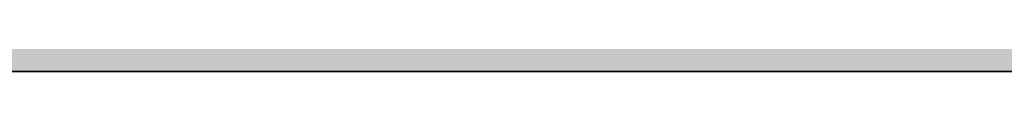
# Model space of a CAD drawing. Units: inches. Extents: x 2083 to 3317, y 1141 to 2115.
# Tile 150 of 256: x 3126.946713 to 3126.955939, y 1263.26136 to 1263.261503. Entities that reach past the tile are written whole.
import ezdxf

# ---------------------------------------------------------------- set-up
doc = ezdxf.new("R2010")
doc.units = ezdxf.units.IN
doc.layers.add('A-ANNO-DIMS', color=2, linetype='Continuous', lineweight=18)
doc.layers.add('A-WALL', color=7, linetype='Continuous', lineweight=35)
doc.layers.add('A-WALL-PATT', color=251, linetype='Continuous', lineweight=13, true_color=0x636466)
doc.styles.get("Standard").update_dxf_attribs({"font": 'arial.ttf'})
doc.dimstyles.new('ISO-25', dxfattribs={"dimtxt": 12, "dimasz": 12, "dimexe": 1.25, "dimexo": 0.625, "dimtad": 1, "dimlunit": 3, "dimtxsty": 'Standard', "dimcen": 2.5, "dimadec": 0, "dimazin": 0, "dimtfac": 1, "dimtmove": 0, "dimatfit": 3, "dimfxl": 1, "dimarcsym": 0})

# ---------------------------------------------------------------- blocks, each defined once
blk = doc.blocks.new('*D10')
at = {"layer": 'A-ANNO-DIMS', "color": 0, "lineweight": -2, "transparency": 16777216}
for p, q in [((2862.9597832, 1262.6363601), (2862.9597832, 1201.3844498)), ((3126.9597832, 1262.6363601), (3126.9597832, 1201.3844498)), ((2874.9597832, 1202.6344498), (3114.9597832, 1202.6344498))]:
    blk.add_line(p, q, dxfattribs=at)
at = {"layer": 'A-ANNO-DIMS', "color": 0, "transparency": 16777216}
for points in [[(2874.9597832, 1204.6344498), (2874.9597832, 1200.6344498), (2862.9597832, 1202.6344498)], [(3114.9597832, 1204.6344498), (3114.9597832, 1200.6344498), (3126.9597832, 1202.6344498)]]:
    blk.add_solid(points, dxfattribs=at)
at = {"layer": 'Defpoints', "color": 0, "transparency": 16777216}
for p in [(2862.9597832, 1263.2613601), (3126.9597832, 1263.2613601), (3126.9597832, 1202.6344498)]:
    blk.add_point(p, dxfattribs=at)
at = {"layer": 'A-ANNO-DIMS', "color": 0, "transparency": 16777216, "insert": (2994.9597832, 1209.2840064), "char_height": 12, "attachment_point": 5}
blk.add_mtext("22'", dxfattribs=at)

msp = doc.modelspace()

# ---------------------------------------------------------------- hatches: boundary and pattern name
at = {"layer": 'A-WALL-PATT'}
h = msp.add_hatch(color=256, dxfattribs=at)
h.dxf.hatch_style = 1
h.paths.add_polyline_path([(3126.9597832, 2020.7613601), (2748.9597832, 2020.7613601), (2604.9597832, 2020.7613601), (2226.9597832, 2020.7613601), (2226.9597832, 1702.7613601), (2466.9597832, 1702.7613601), (2466.9597832, 1582.7613601), (2418.9597832, 1582.7613601), (2418.9597832, 1477.7613601), (2226.9597832, 1477.7613601), (2226.9597832, 1263.2613601), (2544.9597832, 1263.2613601), (2544.9597832, 1411.7613601), (2604.9597832, 1411.7613601), (2685.9597832, 1411.7613601), (2685.9597832, 1420.7613601), (2604.9597832, 1420.7613601), (2604.9597832, 1573.7613601), (2604.9597832, 1702.7613601), (2604.9597832, 2011.7613601), (2748.9597832, 2011.7613601), (2748.9597832, 1702.7613601), (2862.9597832, 1702.7613601), (2862.9597832, 1621.7613601), (2871.9597832, 1621.7613601), (2871.9597832, 1702.7613601), (2883.9597832, 1702.7613601), (2883.9597832, 1706.9394595, -0.026459), (2883.9597832, 1711.7613601), (2757.9597832, 1711.7613601), (2757.9597832, 1807.7613601), (2787.9597832, 1807.7613601), (2787.9597832, 1812.2613601), (2757.9597832, 1812.2613601), (2757.9597832, 2011.7613601), (2877.9597832, 2011.7613601), (2877.9597832, 1812.2613601), (2847.9597832, 1812.2613601), (2847.9597832, 1807.7613601), (2889.8357425, 1807.7613601), (2889.8357425, 1812.2613601), (2882.4597832, 1812.2613601), (2882.4597832, 2011.7613601), (3117.9597832, 2011.7613601), (3117.9597832, 1812.2613601), (2937.8357425, 1812.2613601), (2937.8357425, 1807.7613601), (2995.7097832, 1807.7613601), (2995.7097832, 1796.1176655), (3000.2097832, 1796.1176655), (3000.2097832, 1807.7613601), (3117.9597832, 1807.7613601), (3117.9597832, 1711.7613601), (3000.2097832, 1711.7613601), (3000.2097832, 1760.1176655), (2998.5727047, 1760.1176655, -0.020711), (2995.7097832, 1760.1176655), (2995.7097832, 1711.7613601), (2931.9597832, 1711.7613601), (2931.9597832, 1702.7613601), (3126.9597832, 1702.7613601)])
h.paths.add_polyline_path([(2471.4597832, 2011.7613601), (2471.4597832, 1810.0113601), (2462.7169357, 1810.0113601), (2462.7169357, 1805.5113601), (2505.9597832, 1805.5113601), (2505.9597832, 1810.0113601), (2475.9597832, 1810.0113601), (2475.9597832, 2011.7613601), (2595.9597832, 2011.7613601), (2595.9597832, 1810.0113601), (2565.9597832, 1810.0113601), (2565.9597832, 1805.5113601), (2595.9597832, 1805.5113601), (2595.9597832, 1711.7613601), (2235.9597832, 1711.7613601), (2235.9597832, 1805.5113601), (2353.7097832, 1805.5113601), (2353.7097832, 1796.0541624), (2358.2097832, 1796.0541624), (2358.2097832, 1805.5113601), (2414.7169357, 1805.5113601), (2414.7169357, 1810.0113601), (2235.9597832, 1810.0113601), (2235.9597832, 2011.7613601)], flags=16)
h.paths.add_polyline_path([(2270.2047343, 1994.6100082), (2270.2047343, 1970.6100082), (2246.2047343, 1970.6100082), (2246.2047343, 1994.6100082)], flags=0)
edge = h.paths.add_edge_path(flags=0)
edge.add_ellipse((2332.027391, 1899.7981761), major_axis=(-3.0429938, 3.0429938), ratio=0.16825245, start_angle=-161.3321656, end_angle=-156.3071136, ccw=False)
edge.add_ellipse((2333.0820373, 1898.7435297), major_axis=(-1.0546463, 1.0546463), ratio=0.453532097, start_angle=-123.371019, end_angle=-94.1591066)
edge = h.paths.add_edge_path(flags=0)
edge.add_ellipse((2332.027391, 1968.8762897), major_axis=(3.0429938, 3.0429938), ratio=0.16825245, start_angle=18.6678344, end_angle=23.6928864)
edge.add_spline(control_points=[(2332.9255964, 1970.6911045), (2332.2267681, 1970.3360997), (2330.8937087, 1969.6589054), (2328.4130803, 1970.9321376), (2327.2039345, 1967.7487119), (2324.7095965, 1969.9555886), (2322.5328223, 1967.012354), (2320.0128462, 1971.2958124), (2317.6803077, 1968.1578449), (2316.0405263, 1967.1020468), (2315.4269045, 1966.8096022)], knot_values=[0, 0, 0, 0, 2.267059, 4.324559, 6.685584, 8.878641, 11.121502, 14.300359, 17.755284, 19.732645, 19.732645, 19.732645, 19.732645], degree=3, periodic=0)
edge.add_ellipse((2332.027391, 1968.8762897), major_axis=(3.0429938, 3.0429938), ratio=0.16825245, start_angle=18.6678344, end_angle=23.6928864, ccw=False)
edge.add_ellipse((2333.0820373, 1969.930936), major_axis=(1.0546463, 1.0546463), ratio=0.453532097, start_angle=56.628981, end_angle=85.8408934, ccw=False)
edge = h.paths.add_edge_path(flags=0)
edge.add_spline(control_points=[(2296.4282874, 1967.9879081), (2293.6278045, 1965.3363137), (2287.7036238, 1959.727094), (2299.7438601, 1949.9956993), (2294.5325909, 1935.6685275), (2290.5732281, 1920.6035119), (2293.3941244, 1909.9736911), (2296.1854073, 1904.9665431)], knot_values=[0.099185, 0.099185, 0.099185, 0.099185, 0.345301, 0.619822, 0.982653, 1.386093, 1.810555, 1.810555, 1.810555, 1.810555], degree=3, periodic=0)
edge.add_spline(control_points=[(2296.1854073, 1904.9665431), (2297.3835817, 1902.6193002), (2298.0009694, 1901.9493116), (2298.5529698, 1901.4681549)], knot_values=[0.006246, 0.006246, 0.006246, 0.006246, 0.055476, 0.055476, 0.055476, 0.055476], degree=3, periodic=0)
edge.add_spline(control_points=[(2298.5529698, 1901.4681549), (2297.2586121, 1900.9232238), (2295.2252939, 1900.2321257), (2293.0602287, 1900.6142053), (2292.1014227, 1900.788415), (2292.0895776, 1900.790568)], knot_values=[0.312835, 0.312835, 0.312835, 0.312835, 0.40178, 0.474987, 0.475903, 0.475903, 0.475903, 0.475903], degree=3, periodic=0)
edge.add_arc((2292.7936464, 1904.6641088), 3.9370079, 215.4208969, 259.6981795, ccw=False)
edge.add_spline(control_points=[(2289.5853139, 1902.3823039), (2289.4766524, 1902.5350874), (2289.3684805, 1902.6880353), (2289.2608648, 1902.8411699)], knot_values=[0.102872, 0.102872, 0.102872, 0.102872, 0.116896, 0.116896, 0.116896, 0.116896], degree=3, periodic=0)
edge.add_spline(control_points=[(2289.2608648, 1902.8411699), (2288.6866042, 1902.5501922), (2287.6400477, 1902.0199025), (2285.8813368, 1901.8739536), (2283.8529717, 1901.5043521), (2281.7199871, 1899.7105375), (2278.4669913, 1899.492942), (2276.1571361, 1901.8832022), (2272.2589526, 1899.8040711), (2267.7776054, 1901.8431828), (2262.2438819, 1900.1840326), (2257.414927, 1901.7820606), (2254.318374, 1900.7261196), (2253.1782849, 1900.3373431)], knot_values=[0, 0, 0, 0, 1.907977, 3.477176, 5.261074, 7.972851, 11.680248, 13.717921, 16.939592, 22.789562, 27.502503, 33.595215, 37.145618, 37.145618, 37.145618, 37.145618], degree=3, periodic=0)
edge.add_line((2253.1782849, 1900.3373431), (2250.2442397, 1902.8411699))
edge.add_line((2250.2442397, 1902.8411699), (2250.2442397, 1965.8332959))
edge.add_line((2250.2442397, 1965.8332959), (2253.1782849, 1968.3371226))
edge.add_spline(control_points=[(2253.1782849, 1968.3371226), (2254.318374, 1967.9483462), (2257.414927, 1966.8924051), (2262.2438819, 1968.4904332), (2267.7776054, 1966.8312829), (2271.5267301, 1968.5372172), (2273.8759143, 1967.8282895), (2274.2067012, 1967.7276424)], knot_values=[0, 0, 0, 0, 0.09018, 0.244935, 0.364644, 0.513233, 0.537855, 0.537855, 0.537855, 0.537855], degree=3, periodic=0)
edge.add_arc((2274.3528869, 1963.7933495), 3.9370079, 72.0511336, 92.1279492, ccw=False)
edge.add_arc((2281.2969331, 1985.2300027), 18.5962982, 252.05113361, 288.56572166)
edge.add_arc((2292.3167172, 1956.0288805), 12.6460805, 71.02678788, 113.77821843, ccw=False)
edge = h.paths.add_edge_path(flags=0)
edge.add_spline(control_points=[(2274.8994147, 1951.8561946), (2275.066156, 1951.6165924), (2275.2326866, 1951.3765878), (2275.3979871, 1951.1358545)], knot_values=[1.409916, 1.409916, 1.409916, 1.409916, 1.43159, 1.43159, 1.43159, 1.43159], degree=3, periodic=0)
edge.add_spline(control_points=[(2275.3979871, 1951.1358545), (2275.7921055, 1950.5618854), (2276.1792311, 1949.9837745), (2276.5455462, 1949.3971029)], knot_values=[1.358238, 1.358238, 1.358238, 1.358238, 1.409916, 1.409916, 1.409916, 1.409916], degree=3, periodic=0)
edge.add_line((2276.5455462, 1949.3971029), (2277.437289, 1947.8621847))
edge.add_spline(control_points=[(2277.437289, 1947.8621847), (2276.3038341, 1945.6731147), (2274.6396979, 1942.4268817), (2274.631615, 1938.0938998), (2272.7991237, 1930.8515498), (2274.3564261, 1943.8970461), (2275.9476814, 1947.9233558), (2276.5455462, 1949.3971029)], knot_values=[0.005632, 0.005632, 0.005632, 0.005632, 0.186014, 0.266002, 0.357087, 0.59639, 0.739732, 0.739732, 0.739732, 0.739732], degree=3, periodic=0)
edge.add_spline(control_points=[(2276.5455462, 1949.3971029), (2276.1792311, 1949.9837745), (2275.7921055, 1950.5618854), (2275.3979871, 1951.1358545)], knot_values=[1.358238, 1.358238, 1.358238, 1.358238, 1.409916, 1.409916, 1.409916, 1.409916], degree=3, periodic=0)
edge.add_spline(control_points=[(2275.3979871, 1951.1358545), (2274.9425002, 1950.0804523), (2274.2077604, 1948.0252718), (2273.9346018, 1944.8514774), (2272.4685341, 1937.6274891), (2273.4662155, 1945.6964663), (2274.7006154, 1951.0594725), (2274.8994147, 1951.8561946)], knot_values=[0.104364, 0.104364, 0.104364, 0.104364, 0.189636, 0.269624, 0.36071, 0.600013, 0.644622, 0.644622, 0.644622, 0.644622], degree=3, periodic=0)
h.paths.add_polyline_path([(2269.1675139, 1963.1275729, -0.357527), (2268.170633, 1960.9763695, -0.092561), (2268.170633, 1939.4363249, -0.357527), (2269.1675139, 1937.2851215, -0.357527), (2267.0163105, 1938.2820024, -0.164785), (2254.6855813, 1938.2820024, -0.357527), (2252.5343779, 1937.2851215, -0.357527), (2253.5312587, 1939.4363249, -0.092561), (2253.5312587, 1960.9763695, -0.357527), (2252.5343779, 1963.1275729, -0.357527), (2254.6855813, 1962.130692, -0.164785), (2267.0163105, 1962.130692, -0.357527)], flags=0)
h.paths.add_polyline_path([(2248.8740679, 1967.8017998), (2248.8740679, 1957.0277095), (2249.4577833, 1957.0277095), (2249.4577833, 1911.6467562), (2248.8740679, 1911.6467562), (2248.8740679, 1900.8726659), (2246.5118632, 1900.8726659, 0.197327), (2244.1496584, 1902.4568734), (2244.1496584, 1966.2175923, 0.197327), (2246.5118632, 1967.8017998)], flags=0)
h.paths.add_polyline_path([(2269.1675139, 1931.3893442, -0.357527), (2268.170633, 1929.2381408, -0.092561), (2268.170633, 1907.6980962, -0.357527), (2269.1675139, 1905.5468928, -0.357527), (2267.0163105, 1906.5437737, -0.164785), (2254.6855813, 1906.5437737, -0.357527), (2252.5343779, 1905.5468928, -0.357527), (2253.5312587, 1907.6980962, -0.092561), (2253.5312587, 1929.2381408, -0.357527), (2252.5343779, 1931.3893442, -0.357527), (2254.6855813, 1930.3924634, -0.164785), (2267.0163105, 1930.3924634, -0.357527)], flags=0)
edge = h.paths.add_edge_path(flags=0)
edge.add_spline(control_points=[(2276.1968578, 1906.7237016), (2276.1681442, 1909.0289278), (2276.1140492, 1913.371852), (2270.5984171, 1924.9249783), (2273.9051746, 1919.0127787), (2275.9217115, 1916.2620626), (2275.4745699, 1912.4021495), (2277.2578735, 1910.3806206), (2276.6960436, 1908.2250358), (2276.6462176, 1906.8130226), (2276.6178249, 1906.0084068)], knot_values=[0, 0, 0, 0, 8.61026, 16.221274, 18.843057, 23.804898, 27.440828, 29.356102, 31.203478, 33.650687, 33.650687, 33.650687, 33.650687], degree=3, periodic=0)
edge.add_spline(control_points=[(2276.6178249, 1906.0084068), (2276.6233131, 1905.6241436), (2276.4977381, 1904.6286608), (2275.4417789, 1903.8547251), (2274.9373144, 1903.0804497), (2274.8590804, 1902.8411699)], knot_values=[0.156488, 0.156488, 0.156488, 0.156488, 0.184398, 0.231376, 0.250598, 0.250598, 0.250598, 0.250598], degree=3, periodic=0)
edge.add_line((2274.8590804, 1902.8411699), (2276.50598, 1902.8411699))
edge.add_spline(control_points=[(2276.50598, 1902.8411699), (2276.7883084, 1903.0849395), (2277.6650711, 1904.1251958), (2278.2495378, 1904.340738), (2277.6538719, 1908.5273866), (2278.15567, 1906.2278078), (2278.100464, 1905.2859484), (2278.8466748, 1904.0690054), (2277.8567853, 1903.4149482), (2277.8741909, 1902.9910497), (2277.9035616, 1902.8411699)], knot_values=[0.059574, 0.059574, 0.059574, 0.059574, 0.080753, 0.103741, 0.16972, 0.176036, 0.207137, 0.240474, 0.262341, 0.27366, 0.27366, 0.27366, 0.27366], degree=3, periodic=0)
edge.add_line((2277.9035616, 1902.8411699), (2280.0298255, 1902.8411699))
edge.add_spline(control_points=[(2280.0298255, 1902.8411699), (2279.8882214, 1903.088398), (2279.4992571, 1903.9815512), (2280.1522839, 1905.9393491), (2278.103615, 1909.6577572), (2279.7623946, 1907.185285), (2280.3279002, 1904.8748608), (2280.4851086, 1903.4895904), (2281.4632687, 1903.2494323), (2281.7583431, 1902.9364967), (2281.8340361, 1902.8411699)], knot_values=[0.013856, 0.013856, 0.013856, 0.013856, 0.034874, 0.088867, 0.107879, 0.126738, 0.158714, 0.193757, 0.217487, 0.226722, 0.226722, 0.226722, 0.226722], degree=3, periodic=0)
edge.add_spline(control_points=[(2281.8340361, 1902.8411699), (2281.7875348, 1902.8267029), (2281.6470224, 1902.7829881), (2281.3955272, 1902.85949), (2281.088077, 1902.9852418), (2280.7206826, 1903.060902), (2280.3334513, 1903.0257257), (2280.1247668, 1902.898879), (2280.0298255, 1902.8411699)], knot_values=[0, 0, 0, 0, 0.14413, 0.435517, 0.749276, 1.153046, 1.548371, 1.878348, 1.878348, 1.878348, 1.878348], degree=3, periodic=0)
edge.add_line((2280.0298255, 1902.8411699), (2277.9035616, 1902.8411699))
edge.add_spline(control_points=[(2277.9035616, 1902.8411699), (2277.892855, 1902.7958553), (2277.865396, 1902.6796374), (2277.6074793, 1902.6874828), (2277.2740503, 1902.8006999), (2276.8379209, 1902.6197745), (2276.5838074, 1902.7892611), (2276.50598, 1902.8411699)], knot_values=[0, 0, 0, 0, 0.127189, 0.326199, 0.628009, 1.24357, 1.515331, 1.515331, 1.515331, 1.515331], degree=3, periodic=0)
edge.add_line((2276.50598, 1902.8411699), (2274.8590804, 1902.8411699))
edge.add_spline(control_points=[(2274.8590804, 1902.8411699), (2274.8144367, 1902.8985868), (2274.7251297, 1903.013446), (2274.4934765, 1903.1189684), (2274.2442854, 1902.9605386), (2273.9371207, 1903.1849416), (2273.6140395, 1902.9831428), (2273.4083164, 1902.8830449), (2273.322254, 1902.8411699)], knot_values=[0, 0, 0, 0, 0.21843, 0.436957, 0.687977, 0.990379, 1.398396, 1.69185, 1.69185, 1.69185, 1.69185], degree=3, periodic=0)
edge.add_spline(control_points=[(2273.322254, 1902.8411699), (2273.6167403, 1903.445692), (2274.2739977, 1904.5382529), (2276.0272387, 1904.5737017), (2276.2069634, 1906.5836372), (2276.1968578, 1906.7237016)], knot_values=[0.012227, 0.012227, 0.012227, 0.012227, 0.059472, 0.106218, 0.134458, 0.134458, 0.134458, 0.134458], degree=3, periodic=0)
h.paths.add_polyline_path([(2270.7760538, 1897.7898284), (2270.7760538, 1873.7898284), (2246.7760538, 1873.7898284), (2246.7760538, 1897.7898284)], flags=0)
h.paths.add_polyline_path([(2353.7097832, 1760.0050593), (2353.7097832, 1760.0541624), (2358.2097832, 1760.0541624, -0.033729)], flags=0)
h.paths.add_polyline_path([(2321.8191188, 1737.5291862), (2341.9953271, 1737.5291862, -0.414214), (2343.2032727, 1736.3212406), (2343.2032727, 1721.0205964, -0.414214), (2341.9953271, 1719.8126508), (2321.8191188, 1719.8126508, -0.414214), (2320.6111732, 1721.0205964), (2320.6111732, 1736.3212406, -0.414214)], flags=0)
h.paths.add_polyline_path([(2324.2350099, 1736.3212406), (2339.5794359, 1736.3212406, -0.414214), (2341.9953271, 1733.9053494), (2341.9953271, 1725.4497302, -0.414214), (2339.5794359, 1723.033839), (2333.6805885, 1723.033839), (2333.8453172, 1722.0454666, -0.870646), (2335.4253988, 1721.8258934, -0.767327), (2333.922694, 1721.4232449), (2331.2910241, 1721.4232449, -0.767327), (2329.7883193, 1721.8258934, -0.870646), (2331.3684009, 1722.0454666), (2331.5331296, 1723.033839), (2324.2350099, 1723.033839, -0.414214), (2321.8191188, 1725.4497302), (2321.8191188, 1733.9053494, -0.414214)], flags=0)
h.paths.add_polyline_path([(2570.4837892, 1928.6154443), (2589.6837892, 1928.6154443), (2590.1688286, 1928.6154443), (2590.1688286, 1904.9933971), (2570.4837892, 1904.9933971)], flags=0)
h.paths.add_polyline_path([(2574.4473242, 1927.2638215, -1), (2572.8288357, 1927.2638215, -1)], flags=0)
h.paths.add_polyline_path([(2573.0898665, 1926.9408768), (2573.925032, 1927.7760423), (2574.1477428, 1927.5533315), (2573.3125773, 1926.718166)], flags=0)
h.paths.add_polyline_path([(2578.7790648, 1919.7296175, -1), (2571.5916632, 1919.7296175, -1)], flags=0)
h.paths.add_polyline_path([(2578.385364, 1919.7296175, -1), (2571.985364, 1919.7296175, -1)], flags=0)
h.paths.add_polyline_path([(2331.5957638, 1729.4762156, -1), (2333.6179542, 1729.4762156, -1)], flags=0)
h.paths.add_polyline_path([(2578.0342282, 1927.2638215, -1), (2576.4157396, 1927.2638215, -1)], flags=0)
h.paths.add_polyline_path([(2576.6888513, 1927.5310886), (2576.9115621, 1927.7537993), (2577.7467276, 1926.9186339), (2577.5240168, 1926.6959231)], flags=0)
h.paths.add_polyline_path([(2578.1390648, 1909.8595388, -1), (2572.2316632, 1909.8595388, -1)], flags=0)
h.paths.add_polyline_path([(2577.745364, 1909.8595388, -1), (2572.625364, 1909.8595388, -1)], flags=0)
h.paths.add_polyline_path([(2583.7977179, 1927.2638215, -1), (2582.1792294, 1927.2638215, -1)], flags=0)
h.paths.add_polyline_path([(2582.7186487, 1927.7537993), (2583.5538142, 1926.9186339), (2583.3311034, 1926.6959231), (2582.4959379, 1927.5310886)], flags=0)
h.paths.add_polyline_path([(2582.4959379, 1927.5310886), (2582.7186487, 1927.7537993), (2583.5538142, 1926.9186339), (2583.3311034, 1926.6959231)], flags=0)
h.paths.add_polyline_path([(2587.7390648, 1920.5296175, -1), (2581.8316632, 1920.5296175, -1)], flags=0)
h.paths.add_polyline_path([(2587.345364, 1920.5296175, -1), (2582.225364, 1920.5296175, -1)], flags=0)
h.paths.add_polyline_path([(2587.3846219, 1927.2638215, -1), (2585.7661333, 1927.2638215, -1)], flags=0)
h.paths.add_polyline_path([(2586.0819925, 1926.9802469), (2586.917158, 1927.8154124), (2587.1398688, 1927.5927016), (2586.3047033, 1926.7575361)], flags=0)
h.paths.add_polyline_path([(2588.3790648, 1910.6595388, -1), (2581.1916632, 1910.6595388, -1)], flags=0)
h.paths.add_polyline_path([(2587.985364, 1910.6595388, -1), (2581.585364, 1910.6595388, -1)], flags=0)
h.paths.add_polyline_path([(2417.1677288, 1729.4778955), (2437.3439372, 1729.4778955, -0.414214), (2438.5518828, 1728.2699499), (2438.5518828, 1712.9693057, -0.414214), (2437.3439372, 1711.7613601), (2417.1677288, 1711.7613601, -0.414214), (2415.9597832, 1712.9693057), (2415.9597832, 1728.2699499, -0.414214)], flags=0)
h.paths.add_polyline_path([(2419.58362, 1728.2699499), (2434.928046, 1728.2699499, -0.414214), (2437.3439372, 1725.8540587), (2437.3439372, 1717.3984395, -0.414214), (2434.928046, 1714.9825483), (2429.0291985, 1714.9825483), (2429.1939273, 1713.9941758, -0.870646), (2430.7740089, 1713.7746027, -0.767327), (2429.2713041, 1713.3719542), (2426.6396342, 1713.3719542, -0.767327), (2425.1369294, 1713.7746027, -0.870646), (2426.717011, 1713.9941758), (2426.8817397, 1714.9825483), (2419.58362, 1714.9825483, -0.414214), (2417.1677288, 1717.3984395), (2417.1677288, 1725.8540587, -0.414214)], flags=0)
h.paths.add_polyline_path([(2419.58362, 1728.2699499), (2434.928046, 1728.2699499, -0.414214), (2437.3439372, 1725.8540587), (2437.3439372, 1717.3984395, -0.414214), (2434.928046, 1714.9825483), (2429.0291985, 1714.9825483), (2428.3581177, 1719.0090337), (2427.5528206, 1719.0090337), (2426.8817397, 1714.9825483), (2419.58362, 1714.9825483, -0.414214), (2417.1677288, 1717.3984395), (2417.1677288, 1725.8540587, -0.414214)], flags=0)
h.paths.add_polyline_path([(2426.9443739, 1721.4249248, -1), (2428.9665643, 1721.4249248, -1)], flags=0)
h.paths.add_polyline_path([(2475.9597832, 1702.7613601), (2595.9597832, 1702.7613601), (2595.9597832, 1582.7613601), (2475.9597832, 1582.7613601)], flags=16)
h.paths.add_polyline_path([(2427.9597832, 1573.7613601), (2595.9597832, 1573.7613601), (2595.9597832, 1468.7613601), (2595.9597832, 1420.7613601), (2384.4597832, 1420.7613601), (2384.4597832, 1468.7613601), (2427.9597832, 1468.7613601)], flags=16)
h.paths.add_polyline_path([(2379.9597832, 1468.7613601), (2379.9597832, 1420.7613601), (2235.9597832, 1420.7613601), (2235.9597832, 1468.7613601)], flags=16)
h.paths.add_polyline_path([(2317.8159962, 1466.695767), (2337.9922045, 1466.695767, -0.414214), (2339.2001501, 1465.4878214), (2339.2001501, 1450.1871771, -0.414214), (2337.9922045, 1448.9792315), (2317.8159962, 1448.9792315, -0.414214), (2316.6080506, 1450.1871771), (2316.6080506, 1465.4878214, -0.414214)], flags=0)
h.paths.add_polyline_path([(2320.2318874, 1465.4878214), (2335.5763133, 1465.4878214, -0.414214), (2337.9922045, 1463.0719302), (2337.9922045, 1454.616311, -0.414214), (2335.5763133, 1452.2004198), (2329.6774659, 1452.2004198), (2329.8421946, 1451.2120473, -0.870646), (2331.4222762, 1450.9924742, -0.767327), (2329.9195714, 1450.5898257), (2327.2879015, 1450.5898257, -0.767327), (2325.7851967, 1450.9924742, -0.870646), (2327.3652783, 1451.2120473), (2327.530007, 1452.2004198), (2320.2318874, 1452.2004198, -0.414214), (2317.8159962, 1454.616311), (2317.8159962, 1463.0719302, -0.414214)], flags=0)
h.paths.add_polyline_path([(2320.2318874, 1465.4878214), (2335.5763133, 1465.4878214, -0.414214), (2337.9922045, 1463.0719302), (2337.9922045, 1454.616311, -0.414214), (2335.5763133, 1452.2004198), (2329.6774659, 1452.2004198), (2329.006385, 1456.2269051), (2328.2010879, 1456.2269051), (2327.530007, 1452.2004198), (2320.2318874, 1452.2004198, -0.414214), (2317.8159962, 1454.616311), (2317.8159962, 1463.0719302, -0.414214)], flags=0)
h.paths.add_polyline_path([(2327.5926413, 1458.6427963, -1), (2329.6148317, 1458.6427963, -1)], flags=0)
h.paths.add_polyline_path([(2244.4117436, 1433.3404531), (2241.9209449, 1433.3404531, -0.414214), (2240.0178562, 1435.2435418), (2240.0178562, 1440.9528078, -0.414211), (2241.920925, 1442.8558965), (2244.4117436, 1442.8558965, -1.976472)], flags=0)
h.paths.add_polyline_path([(2245.3568884, 1434.3975358, -0.414214), (2245.3568884, 1441.7988138, -2.144098)], flags=0)
h.paths.add_polyline_path([(2535.9597832, 1416.2613601), (2535.9597832, 1272.2613601), (2235.9597832, 1272.2613601), (2235.9597832, 1416.2613601)], flags=16)
h.paths.add_polyline_path([(2260.1195614, 1384.2928413), (2260.1195614, 1362.0386487), (2237.8653688, 1362.0386487), (2237.8653688, 1384.2928413)], flags=0)
edge = h.paths.add_edge_path(flags=0)
edge.add_line((2318.2518466, 1362.0932983), (2318.1457968, 1362.0009726))
edge.add_ellipse((2317.4451158, 1360.4310442), major_axis=(2.8216404, 2.8216404), ratio=0.16825245, start_angle=18.6678344, end_angle=20.9481273, ccw=False)
edge.add_ellipse((2318.4230451, 1361.4089735), major_axis=(0.9779293, 0.9779293), ratio=0.453532097, start_angle=56.628981, end_angle=70.2262012, ccw=False)
edge = h.paths.add_edge_path(flags=0)
edge.add_line((2319.1073699, 1295.5710784), (2319.0150442, 1295.6771282))
edge.add_ellipse((2317.4451158, 1296.3778091), major_axis=(-2.8216404, 2.8216404), ratio=0.16825245, start_angle=-161.3321656, end_angle=-159.0518727, ccw=False)
edge.add_ellipse((2318.4230451, 1295.3998798), major_axis=(-0.9779293, 0.9779293), ratio=0.453532097, start_angle=-123.371019, end_angle=-109.7737988)
edge = h.paths.add_edge_path(flags=0)
edge.add_spline(control_points=[(2284.2103489, 1301.1702189), (2284.5806878, 1300.444719), (2284.8911891, 1299.8920243), (2285.159553, 1299.4610182)], knot_values=[0.039066, 0.039066, 0.039066, 0.039066, 0.055476, 0.055476, 0.055476, 0.055476], degree=3, periodic=0)
edge.add_line((2285.159553, 1299.4610182), (2284.2103489, 1301.1702189))
edge = h.paths.add_edge_path(flags=0)
edge.add_line((2280.4124579, 1297.2980125), (2283.3699905, 1297.0361216))
edge.add_line((2283.3699905, 1297.0361216), (2286.4056902, 1297.9263104))
edge.add_spline(control_points=[(2286.4056902, 1297.9263104), (2285.305487, 1297.4631193), (2284.3447774, 1297.1291508), (2283.3699905, 1297.0361216)], knot_values=[0.394369, 0.394369, 0.394369, 0.394369, 0.475903, 0.475903, 0.475903, 0.475903], degree=3, periodic=0)
edge.add_spline(control_points=[(2283.3699905, 1297.0361216), (2283.2813895, 1297.027666), (2282.316289, 1296.9573356), (2281.3125019, 1297.1344787), (2280.4234414, 1297.2960161), (2280.4124579, 1297.2980125)], knot_values=[0.312835, 0.312835, 0.312835, 0.312835, 0.320246, 0.393453, 0.394369, 0.394369, 0.394369, 0.394369], degree=3, periodic=0)
edge = h.paths.add_edge_path(flags=0)
edge.add_line((2284.4355615, 1359.6072854), (2280.4462909, 1355.328047))
edge.add_line((2280.4462909, 1355.328047), (2279.5799868, 1351.0177544))
edge.add_line((2279.5799868, 1351.0177544), (2282.4129737, 1346.5804327))
edge.add_spline(control_points=[(2282.4129737, 1346.5804327), (2283.1533308, 1345.5892358), (2284.2528957, 1344.0288973), (2284.801037, 1342.3871671), (2284.9351625, 1341.8055443)], knot_values=[1.240098, 1.240098, 1.240098, 1.240098, 1.332892, 1.382712, 1.382712, 1.382712, 1.382712], degree=3, periodic=0)
edge.add_spline(control_points=[(2284.9351625, 1341.8055443), (2285.3191079, 1340.1406002), (2285.2330291, 1338.4092041), (2284.9099384, 1336.6541222)], knot_values=[1.097484, 1.097484, 1.097484, 1.097484, 1.240098, 1.240098, 1.240098, 1.240098], degree=3, periodic=0)
edge.add_spline(control_points=[(2284.9099384, 1336.6541222), (2284.5868478, 1334.8990403), (2284.0267453, 1333.1202725), (2283.4626437, 1331.3605849)], knot_values=[0.95487, 0.95487, 0.95487, 0.95487, 1.097484, 1.097484, 1.097484, 1.097484], degree=3, periodic=0)
edge.add_line((2283.4626437, 1331.3605849), (2281.8903759, 1326.153357))
edge.add_line((2281.8903759, 1326.153357), (2280.7562592, 1321.0560888))
edge.add_line((2280.7562592, 1321.0560888), (2280.2992048, 1316.0019772))
edge.add_line((2280.2992048, 1316.0019772), (2280.7159327, 1310.9500678))
edge.add_line((2280.7159327, 1310.9500678), (2282.0280939, 1305.9721367))
edge.add_line((2282.0280939, 1305.9721367), (2284.2103489, 1301.1702189))
edge.add_spline(control_points=[(2284.2103489, 1301.1702189), (2283.3407305, 1302.7301854), (2282.6119044, 1304.3364933), (2282.0280939, 1305.9721367)], knot_values=[0.099185, 0.099185, 0.099185, 0.099185, 0.241799, 0.241799, 0.241799, 0.241799], degree=3, periodic=0)
edge.add_spline(control_points=[(2282.0280939, 1305.9721367), (2281.4442835, 1307.6077801), (2281.0054886, 1309.2727591), (2280.7159327, 1310.9500678)], knot_values=[0.241799, 0.241799, 0.241799, 0.241799, 0.384413, 0.384413, 0.384413, 0.384413], degree=3, periodic=0)
edge.add_spline(control_points=[(2280.7159327, 1310.9500678), (2280.4332411, 1312.5876134), (2280.2893863, 1314.2769594), (2280.2988938, 1315.9620324), (2280.2992048, 1316.0019772)], knot_values=[0.384413, 0.384413, 0.384413, 0.384413, 0.523647, 0.527028, 0.527028, 0.527028, 0.527028], degree=3, periodic=0)
edge.add_spline(control_points=[(2280.2992048, 1316.0019772), (2280.3123257, 1317.6869552), (2280.4778706, 1319.3679256), (2280.7562592, 1321.0560888)], knot_values=[0.527028, 0.527028, 0.527028, 0.527028, 0.669642, 0.669642, 0.669642, 0.669642], degree=3, periodic=0)
edge.add_spline(control_points=[(2280.7562592, 1321.0560888), (2281.0346478, 1322.7442519), (2281.4258801, 1324.4396079), (2281.8903759, 1326.153357)], knot_values=[0.669642, 0.669642, 0.669642, 0.669642, 0.812256, 0.812256, 0.812256, 0.812256], degree=3, periodic=0)
edge.add_spline(control_points=[(2281.8903759, 1326.153357), (2282.2643834, 1327.5332507), (2282.7878702, 1329.2618097), (2283.352751, 1331.0177803), (2283.4626437, 1331.3605849)], knot_values=[0.812256, 0.812256, 0.812256, 0.812256, 0.927087, 0.95487, 0.95487, 0.95487, 0.95487], degree=3, periodic=0)
edge.add_line((2283.4626437, 1331.3605849), (2284.9099384, 1336.6541222))
edge.add_line((2284.9099384, 1336.6541222), (2284.9351625, 1341.8055443))
edge.add_line((2284.9351625, 1341.8055443), (2282.4129737, 1346.5804327))
edge.add_spline(control_points=[(2282.4129737, 1346.5804327), (2281.2751273, 1348.1037918), (2280.0784467, 1349.5703178), (2279.5799868, 1351.0177544)], knot_values=[1.382712, 1.382712, 1.382712, 1.382712, 1.525326, 1.525326, 1.525326, 1.525326], degree=3, periodic=0)
edge.add_spline(control_points=[(2279.5799868, 1351.0177544), (2279.4432818, 1351.4147209), (2279.1363124, 1352.856922), (2279.7351897, 1354.2903851), (2280.4462909, 1355.328047)], knot_values=[1.525326, 1.525326, 1.525326, 1.525326, 1.564439, 1.667941, 1.667941, 1.667941, 1.667941], degree=3, periodic=0)
edge.add_spline(control_points=[(2280.4462909, 1355.328047), (2281.4261132, 1356.7578354), (2282.9308373, 1358.1825604), (2284.4355615, 1359.6072854)], knot_values=[1.667941, 1.667941, 1.667941, 1.667941, 1.810555, 1.810555, 1.810555, 1.810555], degree=3, periodic=0)
edge.add_arc((2280.6230749, 1348.518181), 11.7261796, 71.02678788, 113.77821843)
edge.add_arc((2270.4048917, 1375.5951559), 17.2435667, 252.05113361, 288.56572166, ccw=False)
edge.add_arc((2263.9659692, 1355.7178471), 3.6506221, 72.0511336, 92.1279492)
edge.add_arc((2263.9659692, 1355.7178471), 3.6506221, 92.1279492, 177.98513)
edge.add_spline(control_points=[(2260.3176041, 1355.8461989), (2260.2604169, 1354.2206683), (2260.551278, 1350.1865469), (2262.9993445, 1346.7662507), (2264.4727415, 1344.6490245)], knot_values=[1.43159, 1.43159, 1.43159, 1.43159, 1.564144, 1.770695, 1.770695, 1.770695, 1.770695], degree=3, periodic=0)
edge.add_line((2264.4727415, 1344.6490245), (2264.9355904, 1343.9825301))
edge.add_spline(control_points=[(2263.8010444, 1340.2481052), (2263.8432379, 1340.5140884), (2264.0672444, 1341.7564652), (2264.5126928, 1343.0024532), (2264.9350468, 1343.9810834)], knot_values=[0.53657, 0.53657, 0.53657, 0.53657, 0.559349, 0.644622, 0.644622, 0.644622, 0.644622], degree=3, periodic=0)
edge.add_spline(control_points=[(2264.9350468, 1343.9810834), (2265.1177715, 1343.7149747), (2265.2988751, 1343.4479058), (2265.4767562, 1343.1793646)], knot_values=[1.384077, 1.384077, 1.384077, 1.384077, 1.409916, 1.409916, 1.409916, 1.409916], degree=3, periodic=0)
edge.add_spline(control_points=[(2265.4767562, 1343.1793646), (2265.6546373, 1342.9108234), (2265.8292958, 1342.64081), (2265.9991301, 1342.368812)], knot_values=[1.358238, 1.358238, 1.358238, 1.358238, 1.384077, 1.384077, 1.384077, 1.384077], degree=3, periodic=0)
edge.add_line((2265.9991301, 1342.368812), (2266.8260057, 1340.9455468))
edge.add_spline(control_points=[(2266.8260057, 1340.9455468), (2268.894401, 1337.0896912), (2271.3981727, 1325.8430009), (2270.5161644, 1310.5685568), (2275.9193759, 1301.860609), (2277.7895113, 1299.1994495)], knot_values=[0.116896, 0.116896, 0.116896, 0.116896, 0.472987, 1.050969, 1.313793, 1.313793, 1.313793, 1.313793], degree=3, periodic=0)
edge.add_spline(control_points=[(2277.7895113, 1299.1994495), (2277.8394051, 1299.1284519), (2277.8894277, 1299.0574975), (2277.9395717, 1298.9865839)], knot_values=[0.109884, 0.109884, 0.109884, 0.109884, 0.116896, 0.116896, 0.116896, 0.116896], degree=3, periodic=0)
edge.add_line((2277.9395717, 1298.9865839), (2277.7888489, 1299.1991139))
edge.add_spline(control_points=[(2277.7888489, 1299.1991139), (2277.2565819, 1298.9294144), (2276.2863504, 1298.4379024), (2275.0393517, 1298.3344186), (2274.3833299, 1298.2388951), (2274.2152543, 1298.209338)], knot_values=[33.12187, 33.12187, 33.12187, 33.12187, 35.029056, 36.598255, 37.144827, 37.144827, 37.144827, 37.144827], degree=3, periodic=0)
edge.add_line((2274.2152543, 1298.209338), (2273.073147, 1297.8929607))
edge.add_spline(control_points=[(2273.073147, 1297.8929607), (2272.3229363, 1297.579784), (2271.0391507, 1296.5105078), (2269.2483948, 1296.2260622), (2268.4231004, 1296.3746543)], knot_values=[26.532584, 26.532584, 26.532584, 26.532584, 29.198919, 31.839101, 31.839101, 31.839101, 31.839101], degree=3, periodic=0)
edge.add_line((2268.4231004, 1296.3746543), (2263.8785014, 1297.4575338))
edge.add_spline(control_points=[(2263.8785014, 1297.4575338), (2263.5560769, 1297.3594345), (2261.8603064, 1296.8386943), (2260.2387805, 1297.2824073), (2258.9334543, 1297.5164611)], knot_values=[15.919551, 15.919551, 15.919551, 15.919551, 16.939592, 21.226067, 21.226067, 21.226067, 21.226067], degree=3, periodic=0)
edge.add_line((2258.9334543, 1297.5164611), (2254.0552332, 1297.3290098))
edge.add_spline(control_points=[(2254.0552332, 1297.3290098), (2253.7555255, 1297.295815), (2252.1136834, 1297.1651738), (2250.4618687, 1297.5442209), (2249.1296862, 1297.6678818)], knot_values=[5.306517, 5.306517, 5.306517, 5.306517, 6.276435, 10.613034, 10.613034, 10.613034, 10.613034], degree=3, periodic=0)
edge.add_line((2249.1296862, 1297.6678818), (2244.3316495, 1296.8777561))
edge.add_line((2244.3316495, 1296.8777561), (2241.6110326, 1299.1994495))
edge.add_line((2241.6110326, 1299.1994495), (2241.6110326, 1357.6094038))
edge.add_line((2241.6110326, 1357.6094038), (2244.3316495, 1359.9310973))
edge.add_line((2244.3316495, 1359.9310973), (2252.7288228, 1359.5426917))
edge.add_spline(control_points=[(2252.7288228, 1359.5426917), (2252.8709387, 1359.5464396), (2253.3057402, 1359.5481716), (2253.7398447, 1359.5142744), (2254.0317419, 1359.4824261)], knot_values=[0.233291, 0.233291, 0.233291, 0.233291, 0.244935, 0.268927, 0.268927, 0.268927, 0.268927], degree=3, periodic=0)
edge.add_line((2254.0317419, 1359.4824261), (2259.5871899, 1359.4163899))
edge.add_spline(control_points=[(2259.5871899, 1359.4163899), (2260.6770676, 1359.6285026), (2262.0731971, 1359.8970025), (2263.5236925, 1359.4592776), (2263.8304173, 1359.3659518)], knot_values=[0.422516, 0.422516, 0.422516, 0.422516, 0.513233, 0.537855, 0.537855, 0.537855, 0.537855], degree=3, periodic=0)
edge.add_arc((2263.9659692, 1355.7178471), 3.6506221, 72.0511336, 92.1279492, ccw=False)
edge.add_arc((2270.4048917, 1375.5951559), 17.2435667, 252.05113361, 288.56572166)
edge.add_arc((2280.6230749, 1348.518181), 11.7261796, 71.02678788, 113.77821843, ccw=False)
h.paths.add_polyline_path([(2240.3405298, 1359.4347149), (2240.3405298, 1349.4443532), (2240.8817846, 1349.4443532), (2240.8817846, 1307.3645001), (2240.3405298, 1307.3645001), (2240.3405298, 1297.3741385), (2238.1501565, 1297.3741385, 0.197327), (2235.9597832, 1298.8431076), (2235.9597832, 1357.9657458, 0.197327), (2238.1501565, 1359.4347149)], flags=0)
h.paths.add_polyline_path([(2259.1577904, 1355.1005005, -0.357527), (2258.2334246, 1353.1057799, -0.092561), (2258.2334246, 1333.1326007, -0.357527), (2259.1577904, 1331.1378801, -0.357527), (2257.1630698, 1332.0622458, -0.164785), (2245.7293022, 1332.0622458, -0.357527), (2243.7345816, 1331.1378801, -0.357527), (2244.6589474, 1333.1326007, -0.092561), (2244.6589474, 1353.1057799, -0.357527), (2243.7345816, 1355.1005005, -0.357527), (2245.7293022, 1354.1761347, -0.164785), (2257.1630698, 1354.1761347, -0.357527)], flags=0)
edge = h.paths.add_edge_path(flags=0)
edge.add_line((2265.9991301, 1342.368812), (2266.8260057, 1340.9455468))
edge.add_line((2266.8260057, 1340.9455468), (2265.3075567, 1337.8140664))
edge.add_line((2265.3075567, 1337.8140664), (2264.358232, 1334.6529388))
edge.add_line((2264.358232, 1334.6529388), (2264.2620123, 1333.7997046))
edge.add_spline(control_points=[(2264.2620123, 1333.7997046), (2264.2083565, 1333.187055), (2264.1620602, 1332.3655252), (2264.0071444, 1331.4139326), (2263.9690487, 1331.2018338)], knot_values=[0.464444, 0.464444, 0.464444, 0.464444, 0.516691, 0.531608, 0.531608, 0.531608, 0.531608], degree=3, periodic=0)
edge.add_spline(control_points=[(2263.9690487, 1331.2018338), (2263.7745349, 1330.1188727), (2263.4243703, 1328.7908386), (2263.2574202, 1328.5306516), (2263.2340282, 1328.5146115)], knot_values=[0.372682, 0.372682, 0.372682, 0.372682, 0.44885, 0.464444, 0.464444, 0.464444, 0.464444], degree=3, periodic=0)
edge.add_spline(control_points=[(2263.2340282, 1328.5146115), (2263.096382, 1328.4202271), (2263.1311696, 1329.3014765), (2263.2749528, 1330.6157493)], knot_values=[0.280919, 0.280919, 0.280919, 0.280919, 0.372682, 0.372682, 0.372682, 0.372682], degree=3, periodic=0)
edge.add_spline(control_points=[(2263.2749528, 1330.6157493), (2263.4187361, 1331.930022), (2263.6715151, 1333.677318), (2263.9698519, 1335.3150268)], knot_values=[0.189157, 0.189157, 0.189157, 0.189157, 0.280919, 0.280919, 0.280919, 0.280919], degree=3, periodic=0)
edge.add_spline(control_points=[(2263.9698519, 1335.3150268), (2264.1004958, 1336.0321917), (2264.4187827, 1337.6219113), (2264.7548476, 1338.8644304), (2264.9474193, 1339.4911244)], knot_values=[0.097394, 0.097394, 0.097394, 0.097394, 0.137578, 0.189157, 0.189157, 0.189157, 0.189157], degree=3, periodic=0)
edge.add_spline(control_points=[(2264.9474193, 1339.4911244), (2265.2900171, 1340.6060546), (2265.6442376, 1341.4939958), (2265.9991301, 1342.368812)], knot_values=[0.005632, 0.005632, 0.005632, 0.005632, 0.097394, 0.097394, 0.097394, 0.097394], degree=3, periodic=0)
h.paths.add_polyline_path([(2259.1577904, 1325.6709733, -0.357527), (2258.2334246, 1323.6762527, -0.092561), (2258.2334246, 1303.7030735, -0.357527), (2259.1577904, 1301.7083529, -0.357527), (2257.1630698, 1302.6327186, -0.164785), (2245.7293022, 1302.6327186, -0.357527), (2243.7345816, 1301.7083529, -0.357527), (2244.6589474, 1303.7030735, -0.092561), (2244.6589474, 1323.6762527, -0.357527), (2243.7345816, 1325.6709733, -0.357527), (2245.7293022, 1324.7466075, -0.164785), (2257.1630698, 1324.7466075, -0.357527)], flags=0)
edge = h.paths.add_edge_path(flags=0)
edge.add_spline(control_points=[(2261.7089377, 1317.3114208), (2261.6794818, 1317.4175798), (2261.7618581, 1317.3885347), (2262.4907358, 1316.0898725), (2262.962185, 1315.3008975)], knot_values=[14.955861, 14.955861, 14.955861, 14.955861, 16.221274, 18.694826, 18.694826, 18.694826, 18.694826], degree=3, periodic=0)
edge.add_spline(control_points=[(2262.962185, 1315.3008975), (2262.9904374, 1315.2536169), (2263.7020958, 1314.0673762), (2264.3489834, 1313.1271533), (2264.7300545, 1312.1641544)], knot_values=[18.694826, 18.694826, 18.694826, 18.694826, 18.843057, 22.433791, 22.433791, 22.433791, 22.433791], degree=3, periodic=0)
edge.add_spline(control_points=[(2264.7300545, 1312.1641544), (2264.8755649, 1311.7964373), (2265.1768733, 1310.7698073), (2265.1430689, 1309.5592623), (2265.2477363, 1308.8241926)], knot_values=[22.433791, 22.433791, 22.433791, 22.433791, 23.804898, 26.172756, 26.172756, 26.172756, 26.172756], degree=3, periodic=0)
edge.add_line((2265.2477363, 1308.8241926), (2265.8507741, 1307.1718879))
edge.add_spline(control_points=[(2265.8507741, 1307.1718879), (2266.0650246, 1306.8216779), (2266.3843872, 1306.3322461), (2266.4244001, 1305.7805489), (2266.4203688, 1305.6112163)], knot_values=[28.062562, 28.062562, 28.062562, 28.062562, 29.356102, 29.911721, 29.911721, 29.911721, 29.911721], degree=3, periodic=0)
edge.add_spline(control_points=[(2266.4203688, 1305.6112163), (2266.4161162, 1305.4325896), (2266.393999, 1305.2499979), (2266.3647773, 1305.0658571)], knot_values=[29.911721, 29.911721, 29.911721, 29.911721, 30.497837, 30.497837, 30.497837, 30.497837], degree=3, periodic=0)
edge.add_line((2266.3647773, 1305.0658571), (2266.0661511, 1302.1362954))
edge.add_spline(control_points=[(2266.0661511, 1302.1362954), (2266.0712401, 1301.7799843), (2265.9980761, 1301.1999847), (2265.6632664, 1300.7589613), (2265.5089084, 1300.5858824)], knot_values=[0.156488, 0.156488, 0.156488, 0.156488, 0.184398, 0.203543, 0.203543, 0.203543, 0.203543], degree=3, periodic=0)
edge.add_line((2265.5089084, 1300.5858824), (2264.4353411, 1299.1994495))
edge.add_line((2264.4353411, 1299.1994495), (2265.962442, 1299.1994495))
edge.add_line((2265.962442, 1299.1994495), (2267.3359898, 1301.1752758))
edge.add_line((2267.3359898, 1301.1752758), (2267.3116668, 1301.9862366))
edge.add_spline(control_points=[(2267.3116668, 1301.9862366), (2267.261111, 1302.8623959), (2267.1602121, 1303.7371316), (2267.2714865, 1303.3258962)], knot_values=[0.126229, 0.126229, 0.126229, 0.126229, 0.166617, 0.166617, 0.166617, 0.166617], degree=3, periodic=0)
edge.add_spline(control_points=[(2267.2714865, 1303.3258962), (2267.2800347, 1303.2943047), (2267.3097851, 1303.1753659), (2267.3734504, 1302.8836084), (2267.4061233, 1302.6828291), (2267.4179259, 1302.6010251)], knot_values=[0.166617, 0.166617, 0.166617, 0.166617, 0.16972, 0.176036, 0.180765, 0.180765, 0.180765, 0.180765], degree=3, periodic=0)
edge.add_spline(control_points=[(2267.7438914, 1300.9875045), (2267.6875832, 1301.1509426), (2267.4805198, 1301.6566644), (2267.4837514, 1302.1447877), (2267.4179259, 1302.6010251)], knot_values=[0.180765, 0.180765, 0.180765, 0.180765, 0.193767, 0.220139, 0.220139, 0.220139, 0.220139], degree=3, periodic=0)
edge.add_line((2267.4179259, 1302.6010251), (2267.7438914, 1300.9875045))
edge.add_spline(control_points=[(2267.7438914, 1300.9875045), (2267.8319608, 1300.7318778), (2267.9320205, 1300.3099042), (2267.5548409, 1299.9745185), (2267.429366, 1299.8292073)], knot_values=[0.220139, 0.220139, 0.220139, 0.220139, 0.240474, 0.25489, 0.25489, 0.25489, 0.25489], degree=3, periodic=0)
edge.add_line((2267.429366, 1299.8292073), (2267.2583608, 1299.1994495))
edge.add_line((2267.2583608, 1299.1994495), (2269.229956, 1299.1994495))
edge.add_spline(control_points=[(2269.229956, 1299.1994495), (2269.0986525, 1299.4286938), (2268.842774, 1300.0162509), (2269.0115749, 1300.9159235), (2268.9467957, 1301.6607397)], knot_values=[0.013856, 0.013856, 0.013856, 0.013856, 0.034874, 0.067073, 0.067073, 0.067073, 0.067073], degree=3, periodic=0)
edge.add_line((2268.9467957, 1301.6607397), (2268.4315815, 1303.6031089))
edge.add_spline(control_points=[(2268.4315815, 1303.6031089), (2268.1755957, 1304.1923747), (2267.5962136, 1305.2512977), (2268.0406981, 1304.6232098), (2268.2513938, 1304.2824205)], knot_values=[0.090155, 0.090155, 0.090155, 0.090155, 0.107879, 0.120289, 0.120289, 0.120289, 0.120289], degree=3, periodic=0)
edge.add_spline(control_points=[(2268.2513938, 1304.2824205), (2268.3608818, 1304.1053294), (2269.0577527, 1302.9179833), (2269.382691, 1301.5904186), (2269.5214051, 1300.7759312), (2269.5752202, 1300.5557836)], knot_values=[0.120289, 0.120289, 0.120289, 0.120289, 0.126738, 0.158714, 0.173506, 0.173506, 0.173506, 0.173506], degree=3, periodic=0)
edge.add_line((2269.5752202, 1300.5557836), (2270.6857984, 1299.4212579))
edge.add_spline(control_points=[(2270.6857984, 1299.4212579), (2270.7672206, 1299.3572512), (2270.8378523, 1299.2814011), (2270.9029248, 1299.1994495)], knot_values=[0.21816, 0.21816, 0.21816, 0.21816, 0.226722, 0.226722, 0.226722, 0.226722], degree=3, periodic=0)
edge.add_line((2270.9372012, 1299.1929131), (2270.9029248, 1299.1994495))
edge.add_spline(control_points=[(2270.9029248, 1299.1994495), (2270.8598061, 1299.1860349), (2270.7295148, 1299.1455), (2270.4963139, 1299.216437), (2270.2716612, 1299.3083234), (2270.1210168, 1299.3479612), (2270.0633386, 1299.3595566)], knot_values=[0.939174, 0.939174, 0.939174, 0.939174, 1.083304, 1.374691, 1.68845, 1.878348, 1.878348, 1.878348, 1.878348], degree=3, periodic=0)
edge.add_line((2270.0633386, 1299.3595566), (2269.229956, 1299.1994495))
edge.add_line((2269.229956, 1299.1994495), (2267.2583608, 1299.1994495))
edge.add_spline(control_points=[(2267.2583608, 1299.1994495), (2267.248433, 1299.1574312), (2267.2229714, 1299.0496673), (2266.9838161, 1299.056942), (2266.8092097, 1299.1162303), (2266.6769047, 1299.1090913), (2266.636531, 1299.1048147)], knot_values=[0.757665, 0.757665, 0.757665, 0.757665, 0.884854, 1.083864, 1.385675, 1.515331, 1.515331, 1.515331, 1.515331], degree=3, periodic=0)
edge.add_spline(control_points=[(2266.636531, 1299.1048147), (2266.4852248, 1299.0887878), (2266.2358066, 1299.0171229), (2266.0346081, 1299.1513168), (2265.962442, 1299.1994495)], knot_values=[0, 0, 0, 0, 0.485905, 0.757665, 0.757665, 0.757665, 0.757665], degree=3, periodic=0)
edge.add_line((2265.962442, 1299.1994495), (2264.4353411, 1299.1994495))
edge.add_line((2264.4353411, 1299.1994495), (2263.8584442, 1299.3671176))
edge.add_spline(control_points=[(2263.8584442, 1299.3671176), (2263.8189433, 1299.3709053), (2263.7795277, 1299.3857212), (2263.7401308, 1299.4015039)], knot_values=[0.845925, 0.845925, 0.845925, 0.845925, 0.978627, 0.978627, 0.978627, 0.978627], degree=3, periodic=0)
edge.add_line((2263.7217862, 1299.3964251), (2263.0103065, 1299.1994495))
edge.add_spline(control_points=[(2263.0103065, 1299.1994495), (2263.2457942, 1299.682859), (2263.5060317, 1300.1281072), (2263.8734943, 1300.4080279)], knot_values=[0.012227, 0.012227, 0.012227, 0.012227, 0.052971, 0.052971, 0.052971, 0.052971], degree=3, periodic=0)
edge.add_spline(control_points=[(2263.8734943, 1300.4080279), (2263.932131, 1300.4526954), (2264.0842429, 1300.5529789), (2264.2551889, 1300.6242227), (2264.3596855, 1300.6647475)], knot_values=[0.052971, 0.052971, 0.052971, 0.052971, 0.059472, 0.069086, 0.069086, 0.069086, 0.069086], degree=3, periodic=0)
edge.add_line((2264.3596855, 1300.6647475), (2265.1418998, 1301.0777737))
edge.add_line((2265.1418998, 1301.0777737), (2265.675806, 1302.7995583))
edge.add_line((2265.675806, 1302.7995583), (2265.5407004, 1305.7040662))
edge.add_line((2265.5407004, 1305.7040662), (2264.8030733, 1309.3277237))
edge.add_line((2264.8030733, 1309.3277237), (2263.0405349, 1314.0917906))
edge.add_spline(control_points=[(2263.0405349, 1314.0917906), (2262.3835724, 1315.6714379), (2261.7959724, 1316.9977489), (2261.7089377, 1317.3114208)], knot_values=[11.216896, 11.216896, 11.216896, 11.216896, 14.955861, 14.955861, 14.955861, 14.955861], degree=3, periodic=0)
h.paths.add_polyline_path([(2871.9597832, 1416.2613601), (2895.910047, 1416.2613601), (2895.910047, 1420.7613601), (2871.9597832, 1420.7613601), (2871.9597832, 1501.7613601), (2862.9597832, 1501.7613601), (2862.9597832, 1420.7613601), (2805.9597832, 1420.7613601), (2805.9597832, 1411.7613601), (2862.9597832, 1411.7613601), (2862.9597832, 1263.2613601), (3126.9597832, 1263.2613601), (3126.9597832, 1411.7613601), (3126.9597832, 1486.7613601), (2943.9597832, 1486.7613601), (2943.9597832, 1477.7613601), (2967.8603109, 1477.7613601), (2967.8603109, 1420.7613601), (2943.910047, 1420.7613601), (2943.910047, 1416.2613601), (3117.9597832, 1416.2613601), (3117.9597832, 1420.7613601), (2972.3603109, 1420.7613601), (2972.3603109, 1477.7613601), (3117.9597832, 1477.7613601), (3117.9597832, 1420.7613601), (3117.9597832, 1272.2613601), (2871.9597832, 1272.2613601)], flags=0)
h.paths.add_polyline_path([(2457.1256256, 1485.9425054), (2527.6026508, 1485.9425054), (2527.6026508, 1537.6357021), (2457.1256256, 1537.6357021)], flags=8)
h.paths.add_polyline_path([(2481.0050583, 1609.9818039), (2590.765818, 1609.9818039), (2590.765818, 1682.0033623), (2481.0050583, 1682.0033623)], flags=8)
h.paths.add_polyline_path([(2483.0850224, 1729.1267835), (2553.5620476, 1729.1267835), (2553.5620476, 1780.8199802), (2483.0850224, 1780.8199802)], flags=8)
h = msp.add_hatch(color=256, dxfattribs=at)
h.dxf.hatch_style = 1
h.paths.add_polyline_path([(3126.9597832, 1486.7613601), (2943.9597832, 1486.7613601), (2943.9597832, 1477.7613601), (2967.8603109, 1477.7613601), (2967.8603109, 1420.7613601), (2943.910047, 1420.7613601), (2943.910047, 1416.2613601), (3117.9597832, 1416.2613601), (3117.9597832, 1420.7613601), (2972.3603109, 1420.7613601), (2972.3603109, 1477.7613601), (3117.9597832, 1477.7613601), (3117.9597832, 1420.7613601), (3117.9597832, 1272.2613601), (2871.9597832, 1272.2613601), (2871.9597832, 1416.2613601), (2895.910047, 1416.2613601), (2895.910047, 1420.7613601), (2871.9597832, 1420.7613601), (2871.9597832, 1501.7613601), (2862.9597832, 1501.7613601), (2862.9597832, 1420.7613601), (2805.9597832, 1420.7613601), (2805.9597832, 1411.7613601), (2862.9597832, 1411.7613601), (2862.9597832, 1263.2613601), (3126.9597832, 1263.2613601), (3126.9597832, 1411.7613601)])

# ---------------------------------------------------------------- linework, layer by layer
at = {"layer": 'A-WALL'}
msp.add_line((2544.9597832, 1263.2613601), (3126.9597832, 1263.2613601), dxfattribs=at)

# ---------------------------------------------------------------- dimensions: what is measured, and where the dimension line sits
at = {"layer": 'A-ANNO-DIMS'}
dim = msp.add_linear_dim(base=(3126.9597832, 1202.6344498), p1=(2862.9597832, 1263.2613601), p2=(3126.9597832, 1263.2613601), dimstyle='ISO-25', override={"dimclrd": 0, "dimclre": 0, "dimclrt": 0}, dxfattribs=at)
dim.commit()
dim.dimension.update_dxf_attribs({"geometry": '*D10', "text_midpoint": (2994.9597832, 1209.2840064)})

doc.saveas('drawing.dxf')
